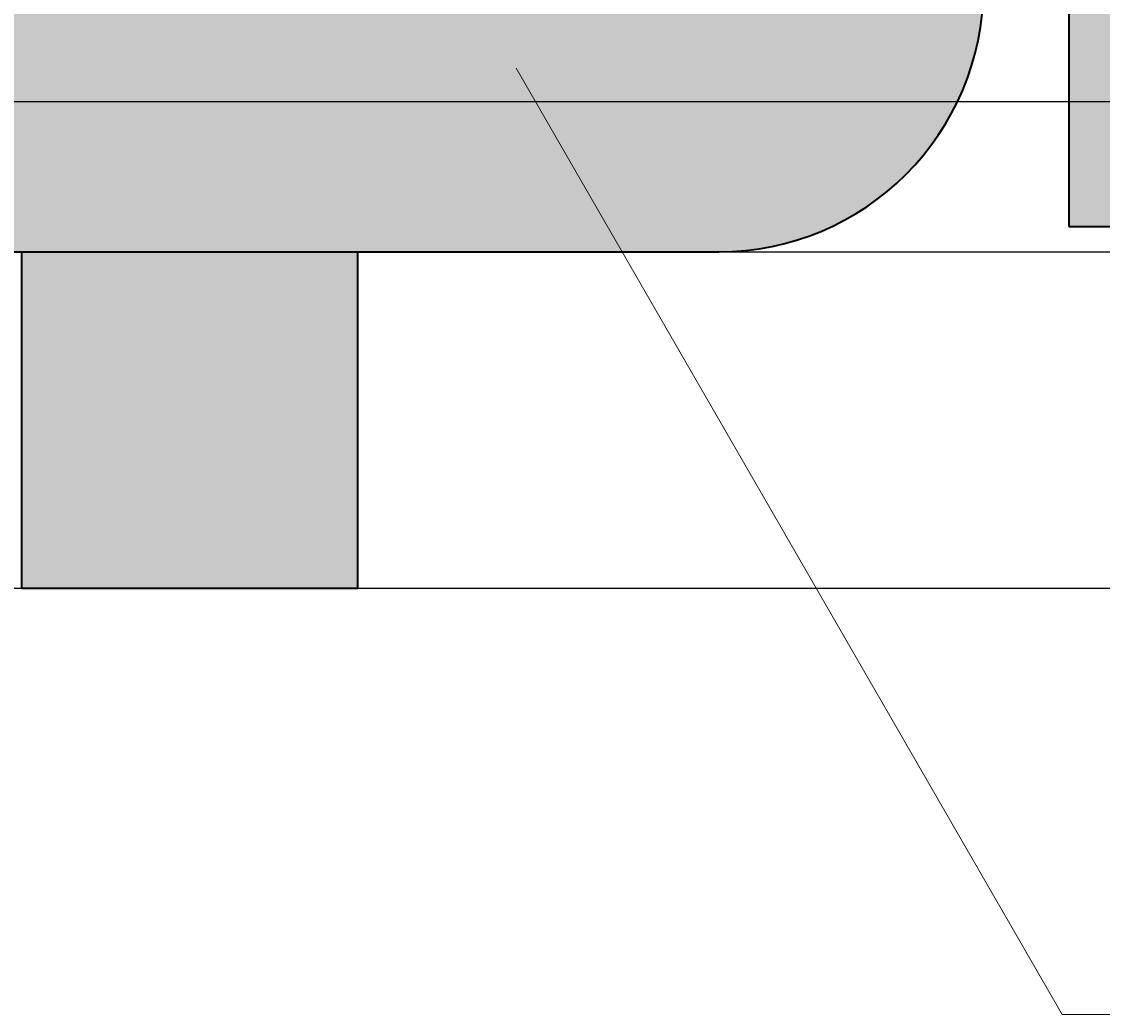
# Model space of a CAD drawing. Units: inches. Extents: x -1 to 292, y -3 to 199.
# Tile 18 of 52: x 148 to 181, y 13 to 42. Entities that reach past the tile are written whole.
import ezdxf

# ---------------------------------------------------------------- set-up
doc = ezdxf.new("R2010")
doc.units = ezdxf.units.IN
doc.header["$MEASUREMENT"] = 0
for name, color, linetype, lineweight in [('M-ANNO-LEAD', 2, 'Continuous', 18), ('M-DIMS', 2, 'Continuous', 18), ('M-EQPM', 7, 'Continuous', 35), ('M-PATT', 8, 'Continuous', 13)]:
    doc.layers.add(name, color=color, linetype=linetype, lineweight=lineweight)
doc.styles.get("Standard").update_dxf_attribs({"font": 'arial.ttf'})
doc.dimstyles.get("Standard").update_dxf_attribs({"dimtxt": 0.18, "dimasz": 0.18, "dimexe": 0.18, "dimexo": 0.0625, "dimgap": 0.09, "dimtad": 0, "dimtih": 1, "dimtoh": 1, "dimdec": 4, "dimzin": 0, "dimdsep": 46, "dimtxsty": 'Standard', "dimcen": 0.09, "dimadec": 0, "dimazin": 0, "dimtfac": 1, "dimtdec": 4, "dimtofl": 0, "dimtmove": 0, "dimatfit": 3, "dimfxl": 1, "dimtolj": 1, "dimtzin": 0, "dimarcsym": 0})

# ---------------------------------------------------------------- blocks, each defined once
blk = doc.blocks.new('SADDLE-SUPPORT')
for p, q in [((0, 10), (0, 0)), ((10, 0), (10, 10)), ((0, 0), (10, 0))]:
    blk.add_line(p, q)
blk = doc.blocks.new('*D7')
at = {"layer": 'Defpoints', "color": 0, "transparency": 16777216}
for p in [(21.861, 54.582), (205.115, 54.582), (21.861, 39.982)]:
    blk.add_point(p, dxfattribs=at)
at = {"layer": 'M-DIMS', "color": 0, "lineweight": -2, "transparency": 16777216}
for p, q in [((21.861, 54.52), (21.861, 39.802)), ((205.115, 54.52), (205.115, 39.802)), ((22.041, 39.982), (113.033, 39.982)), ((204.935, 39.982), (113.944, 39.982))]:
    blk.add_line(p, q, dxfattribs=at)
at = {"layer": 'M-DIMS', "color": 0, "transparency": 16777216}
for points in [[(22.041, 40.012), (22.041, 39.952), (21.861, 39.982)], [(204.935, 40.012), (204.935, 39.952), (205.115, 39.982)]]:
    blk.add_solid(points, dxfattribs=at)
at = {"layer": 'M-DIMS', "color": 0, "transparency": 16777216, "insert": (113.488, 39.982), "char_height": 0.18, "attachment_point": 5}
blk.add_mtext('\\A1;183.25', dxfattribs=at)
blk = doc.blocks.new('*D11')
at = {"layer": 'Defpoints', "color": 0, "transparency": 16777216}
for p in [(79.013, 35.514), (292.04, 35.514), (79.013, 25.514)]:
    blk.add_point(p, dxfattribs=at)
at = {"layer": 'M-DIMS', "color": 0, "lineweight": -2, "transparency": 16777216}
for p, q in [((79.076, 35.514), (292.22, 35.514)), ((292.04, 35.334), (292.04, 30.696)), ((292.04, 25.694), (292.04, 30.332)), ((79.076, 25.514), (292.22, 25.514))]:
    blk.add_line(p, q, dxfattribs=at)
at = {"layer": 'M-DIMS', "color": 0, "transparency": 16777216}
for points in [[(292.01, 35.334), (292.07, 35.334), (292.04, 35.514)], [(292.01, 25.694), (292.07, 25.694), (292.04, 25.514)]]:
    blk.add_solid(points, dxfattribs=at)
at = {"layer": 'M-DIMS', "color": 0, "transparency": 16777216, "insert": (292.04, 30.514), "char_height": 0.18, "attachment_point": 5}
blk.add_mtext('\\A1;10', dxfattribs=at)

msp = doc.modelspace()

# ---------------------------------------------------------------- hatches: boundary and pattern name
at = {"layer": 'M-PATT'}
h = msp.add_hatch(color=256, dxfattribs=at)
h.set_gradient(color1=(0, 127, 0), color2=(0, 127, 0), tint=1, name='CYLINDER')
h.paths.add_polyline_path([(164.5186, 119.2985), (129.9293, 119.2985), (129.9293, 117.2985), (164.1897, 117.2985)])
h.paths.add_polyline_path([(181.5897, 119.2985), (164.5186, 119.2985), (164.1897, 117.2985), (179.5897, 117.2985), (179.5897, 107.8518), (181.5897, 109.1506)])
h.paths.add_polyline_path([(181.5897, 109.1506), (179.5897, 107.8518), (179.5897, 36.2698), (198.4159, 36.2698), (198.4159, 38.2698), (181.5897, 38.2698)])
h.paths.add_polyline_path([(115.4883, 126.765), (111.4883, 126.765), (111.4883, 114.6589), (115.4883, 114.6589)])
h.paths.add_polyline_path([(123.408, 119.2985), (115.4883, 119.2985), (115.4883, 117.2985), (123.408, 117.2985)])
h.paths.add_polyline_path([(115.4883, 112.6589), (111.4883, 112.6589), (111.4883, 106.9941), (115.4883, 106.9941)])
h.paths.add_polyline_path([(120.9032, 106.9941), (106.0735, 106.9941), (106.0735, 105.9941), (120.9032, 105.9941)])
h.paths.add_polyline_path([(236.4209, 117.5104), (234.9209, 117.5104), (234.9209, 97.1861), (236.4209, 97.1861)])
h.paths.add_polyline_path([(236.4209, 126.4904), (234.9209, 126.4904), (234.9209, 118.9331), (236.4209, 118.9331)])
h.paths.add_polyline_path([(244.9552, 125.7269), (242.9552, 125.7269), (242.9552, 116.8562), (244.9552, 116.8562)])
h.paths.add_polyline_path([(244.9552, 115.1721), (242.9552, 115.1721), (242.9552, 109.7385), (244.9552, 109.7385)])
h.paths.add_polyline_path([(248.4468, 109.7385), (239.4637, 109.7385), (239.4637, 109.4289), (248.4468, 109.4289)])
h = msp.add_hatch(color=256, dxfattribs=at)
h.set_gradient(color1=(0, 255, 255), color2=(0, 255, 255), tint=1)
h.paths.add_polyline_path([(75.3521, 99.7735), (72.66, 101.3278), (70.2665, 99.7735), (67.5744, 101.3278), (65.1809, 99.7735), (62.4888, 101.3278), (60.0953, 99.7735), (57.4032, 101.3278), (55.0097, 99.7735), (52.3176, 101.3278), (49.9241, 99.7735, 0.4142136), (57.8007, 91.897), (61.6788, 91.897), (61.6788, 51.2672), (57.8007, 51.2672, 0.8088808), (54.5813, 36.2021), (65.0947, 51.2672), (64.6788, 51.2672), (64.6788, 91.897), (67.6788, 91.897), (67.6788, 51.2672), (65.0947, 51.2672), (54.5813, 36.2021, 0.1056561), (57.8007, 35.5141), (169.176, 35.5141, 1), (169.176, 51.2672), (162.6788, 51.2672), (162.6788, 91.897), (169.176, 91.897, 0.4144629), (177.0526, 99.7802), (174.372, 101.3278), (171.9786, 99.7735), (169.2864, 101.3278), (166.893, 99.7735), (164.2008, 101.3278), (162.1623, 100.004), (162.1623, 96.1027), (160.6222, 96.1027), (160.6222, 100.4578), (159.1152, 101.3278), (156.7218, 99.7735), (154.0296, 101.3278), (151.6362, 99.7735), (148.944, 101.3278), (146.5506, 99.7735), (143.8584, 101.3278), (141.465, 99.7735), (138.7728, 101.3278), (136.3794, 99.7735), (133.6872, 101.3278), (131.2938, 99.7735), (128.6016, 101.3278), (126.2082, 99.7735), (123.516, 101.3278), (121.1225, 99.7735), (118.4304, 101.3278), (116.0369, 99.7735), (113.3448, 101.3278), (110.9513, 99.7735), (108.2592, 101.3278), (105.8657, 99.7735), (103.1736, 101.3278), (100.7801, 99.7735), (98.088, 101.3278), (95.6945, 99.7735), (93.0024, 101.3278), (90.6089, 99.7735), (87.9168, 101.3278), (85.5233, 99.7735), (82.8312, 101.3278), (80.4377, 99.7735), (77.7456, 101.3278)])
h.paths.add_polyline_path([(79.6788, 91.897), (79.6788, 51.2672), (76.6788, 51.2672), (76.6788, 91.897)], flags=16)
h.paths.add_polyline_path([(73.6788, 91.897), (73.6788, 51.2672), (70.6788, 51.2672), (70.6788, 91.897)], flags=16)
h.paths.add_polyline_path([(82.6788, 91.897), (101.6788, 91.897), (101.6788, 51.2672), (82.6788, 51.2672)], flags=16)
h.paths.add_polyline_path([(104.6788, 91.897), (107.6788, 91.897), (107.6788, 51.2672), (104.6788, 51.2672)], flags=16)
h.paths.add_polyline_path([(110.6788, 91.897), (113.6788, 91.897), (113.6788, 51.2672), (110.6788, 51.2672)], flags=16)
h.paths.add_polyline_path([(116.6788, 91.897), (119.6788, 91.897), (119.6788, 51.2672), (116.6788, 51.2672)], flags=16)
h.paths.add_polyline_path([(122.6788, 91.897), (141.6788, 91.897), (141.6788, 51.2672), (144.6788, 51.2672), (144.6788, 91.897), (147.6788, 91.897), (147.6788, 51.2672), (122.6788, 51.2672)], flags=16)
h.paths.add_polyline_path([(150.6788, 91.897), (153.6788, 91.897), (153.6788, 51.2672), (150.6788, 51.2672)], flags=16)
h.paths.add_polyline_path([(156.6788, 91.897), (159.6788, 91.897), (159.6788, 51.2672), (156.6788, 51.2672)], flags=16)
h = msp.add_hatch(color=256, dxfattribs=at)
h.set_gradient(color1=(128, 128, 128), color2=(192, 192, 192), tint=1, name='CYLINDER')
h.paths.add_polyline_path([(158.4295, 25.5141), (158.4295, 35.5141), (148.4295, 35.5141), (148.4295, 25.5141)])
h.paths.add_polyline_path([(79.013, 25.5141), (79.013, 35.5141), (69.013, 35.5141), (69.013, 25.5141)])
h.paths.add_polyline_path([(253.2006, 30.7296), (249.5623, 37.0313, -0.2494892), (240.7896, 35.6769), (237.9333, 30.7296)])

# ---------------------------------------------------------------- linework, layer by layer
at = {"layer": 'M-ANNO-LEAD'}
for p, q in [((163.1424, 40.9785), (179.3919, 12.8335)), ((179.3919, 12.8335), (185.4506, 12.8335))]:
    msp.add_line(p, q, dxfattribs=at)
at = {"layer": 'M-EQPM'}
msp.add_line((179.5897, 36.2698), (198.4159, 36.2698), dxfattribs=at)
msp.add_lwpolyline([(129.9293, 117.2985), (179.5897, 117.2985), (179.5897, 36.2698)], dxfattribs=at)
msp.add_lwpolyline([(61.6788, 51.2672), (57.8007, 51.2672, 1), (57.8007, 35.5141), (169.176, 35.5141, 1), (169.176, 51.2672), (162.6788, 51.2672)], format="xyb", dxfattribs=at)

# ---------------------------------------------------------------- block references
msp.add_blockref('SADDLE-SUPPORT', (148.4294, 25.514), dxfattribs=at)

# ---------------------------------------------------------------- dimensions: what is measured, and where the dimension line sits
at = {"layer": 'M-DIMS'}
for base, p1, p2, angle, override, picture, middle in [((21.8612, 39.9821), (205.1155, 54.5821), (21.8612, 54.5821), 180, {"dimdec": 2, "dimlfac": 1, "dimrnd": 0, "dimzin": 0, "dimdsep": 46, "dimlunit": 2}, '*D7', (113.4883, 39.9821)), ((292.0399, 35.5141), (79.013, 25.5141), (79.013, 35.5141), 90, {"dimdec": 0, "dimlfac": 1, "dimrnd": 0, "dimzin": 0, "dimdsep": 46, "dimlunit": 2}, '*D11', (292.0399, 30.5141))]:
    dim = msp.add_linear_dim(base=base, p1=p1, p2=p2, angle=angle, dimstyle='Standard', override=override, dxfattribs=at)
    dim.commit()
    dim.dimension.update_dxf_attribs({"geometry": picture, "text_midpoint": middle})

doc.saveas('drawing.dxf')
